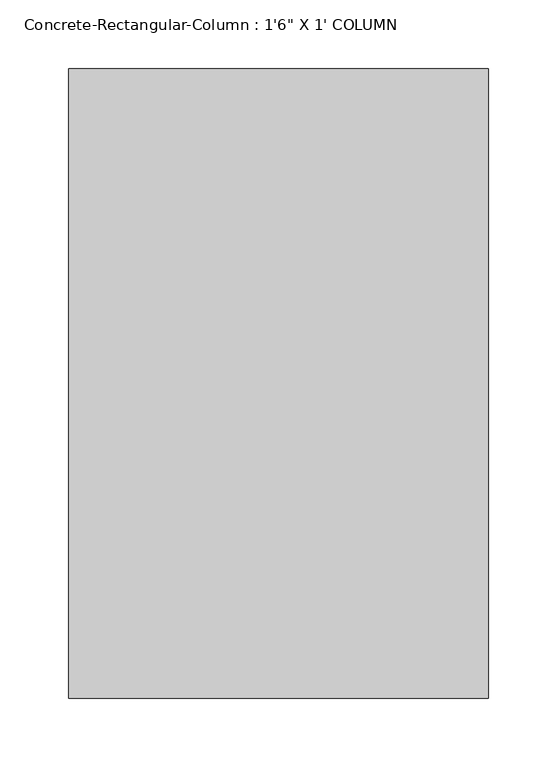
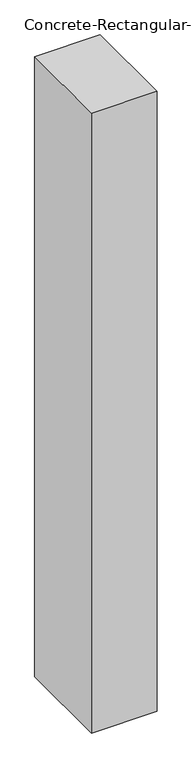
"""IFC4 building model written with IfcOpenShell, lengths in millimetres: column geometry."""

from ifc_helpers import new_model, si_unit, frame, origin, place, context, project, spatial, polyline, outline, extrude, source, transform, mapped, element, save


def column_11789f6a(model_context):
    return source(origin(), model_context, "Body", "SweptSolid", [
        extrude(outline(polyline([(152.4, 228.6), (152.4, -228.6), (-152.4, -228.6), (-152.4, 228.6), (152.4, 228.6)])), frame((0.0, 0.0, 3352.8), z_axis=(0.0, 0.0, 1.0), x_axis=(1.0, 0.0, 0.0)), (0.0, 0.0, 1.0), 3048.0),
    ])


if __name__ == "__main__":
    model = new_model("IFC4")
    model_context = context("Model", 3, world=origin())
    ifc_project = project(units=[si_unit("LENGTHUNIT", "METRE", prefix="MILLI")], contexts=[model_context])
    site = spatial("IfcSite", under=ifc_project)
    building = spatial("IfcBuilding", under=site)
    placement = place(None, origin())
    column_shape = column_11789f6a(model_context)
    element("IfcColumn", 1, ObjectType="Concrete-Rectangular-Column : 1'6\" X 1' COLUMN", at=placement, inside=building, context=model_context, shape_type="MappedRepresentation", body=[
        mapped(column_shape, transform((0.0, 0.0, 0.0), x_axis=(1.0, 0.0, 0.0), y_axis=(0.0, 1.0, 0.0), z_axis=(0.0, 0.0, 1.0))),
    ])
    save(model, "model.ifc")

# Revit data of these elements
# Type "Concrete-Rectangular-Column : 1'6\" X 1' COLUMN"
#   Assembly Code = "B10"
#   b = 1' - 0"
#   h = 1' - 6"
#   Structural Material [instance default] = Concrete, Cast-in-Place gray
# Element 1 (IfcColumn, "Concrete-Rectangular-Column : 1'6\" X 1' COLUMN")
#   Structural Material = WARM BEIGE COLOUR
#   Materials on its faces: "WARM BEIGE COLOUR"
# Materials
#   "Concrete, Cast-in-Place gray": class "Concrete", colour RGB 192 192 192, transparency 0, Description = "Cast-in-place concrete", Cost = 0
#   "WARM BEIGE COLOUR": class "Generic", colour RGB 120 120 120, transparency 0, Cost = 0
